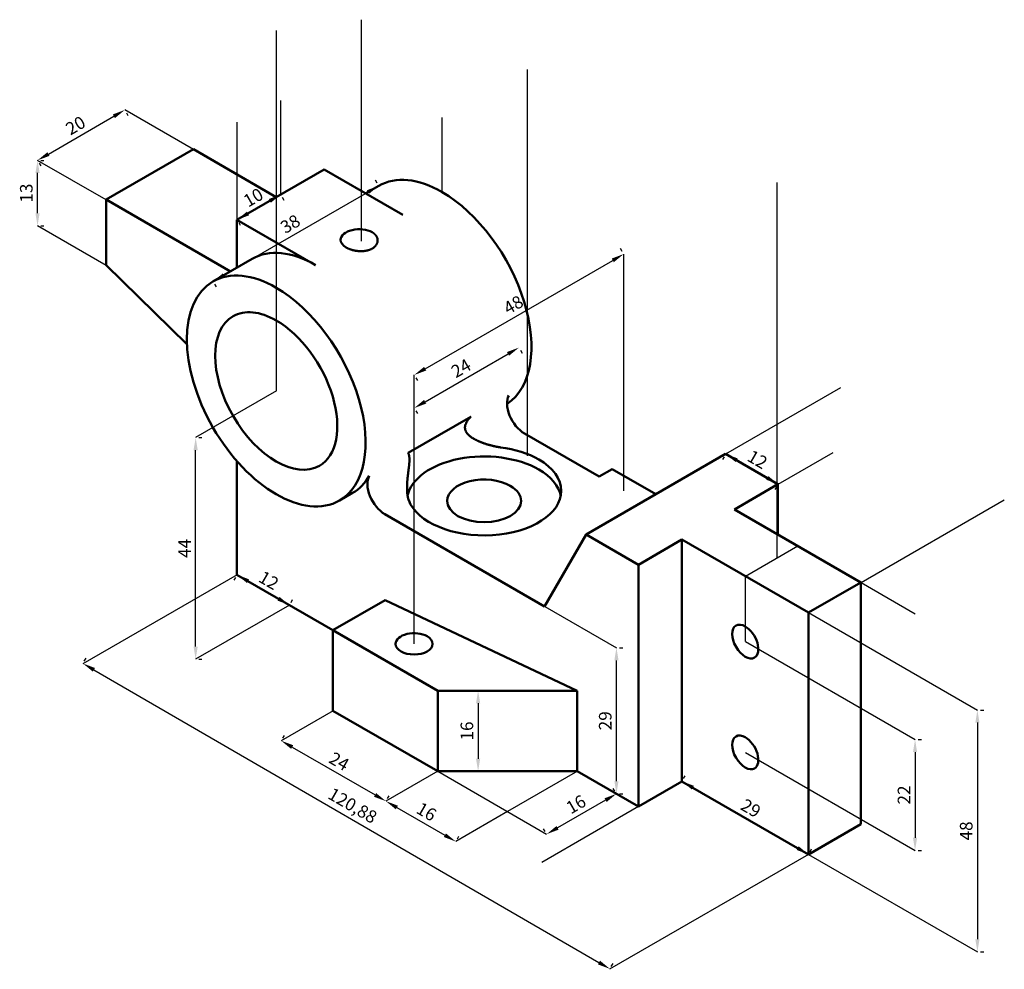
# Model space of a CAD drawing. Units: millimetres. Extents: x 3904 to 4099, y 5304 to 5492.
import ezdxf

# ---------------------------------------------------------------- set-up
doc = ezdxf.new("R2010")
doc.units = ezdxf.units.MM
doc.layers.add('M-DIMS', color=2, linetype='Continuous', lineweight=25)
doc.layers.add('M-OUTL', color=7, linetype='Continuous', lineweight=50)
doc.styles.get("Standard").update_dxf_attribs({"font": 'arial.ttf'})
doc.dimstyles.new('ISO-25', dxfattribs={"dimtxt": 2.5, "dimasz": 2.5, "dimexe": 1.25, "dimexo": 0.625, "dimtad": 1, "dimtxsty": 'Standard', "dimcen": 2.5, "dimadec": 0, "dimazin": 0, "dimtfac": 1, "dimtmove": 0, "dimatfit": 3, "dimfxl": 1, "dimarcsym": 0})

# ---------------------------------------------------------------- blocks, each defined once
blk = doc.blocks.new('*D1')
at = {"layer": 'Defpoints', "color": 0, "transparency": 16777216}
for p in [(4022.48, 5367.43), (4022.48, 5367.43), (4022.48, 5338.43)]:
    blk.add_point(p, dxfattribs=at)
at = {"layer": 'M-DIMS', "color": 0, "lineweight": -2, "transparency": 16777216}
for p, q in [((4023.11, 5367.43), (4023.73, 5367.43)), ((4022.48, 5340.93), (4022.48, 5364.93)), ((4023.11, 5338.43), (4023.73, 5338.43))]:
    blk.add_line(p, q, dxfattribs=at)
at = {"layer": 'M-DIMS', "color": 0, "transparency": 16777216}
for points in [[(4022.07, 5364.93), (4022.9, 5364.93), (4022.48, 5367.43)], [(4022.07, 5340.93), (4022.9, 5340.93), (4022.48, 5338.43)]]:
    blk.add_solid(points, dxfattribs=at)
at = {"layer": 'M-DIMS', "color": 0, "transparency": 16777216, "insert": (4020.58, 5352.93), "char_height": 2.5, "attachment_point": 5, "rotation": 90}
blk.add_mtext('29', dxfattribs=at)
blk = doc.blocks.new('*D2')
at = {"layer": 'Defpoints', "color": 0, "transparency": 16777216}
for p in [(3995.02, 5358.9), (3995.02, 5342.9), (3995.02, 5342.9)]:
    blk.add_point(p, dxfattribs=at)
at = {"layer": 'M-DIMS', "color": 0, "lineweight": -2, "transparency": 16777216}
for p, q in [((3995.65, 5358.9), (3996.27, 5358.9)), ((3995.02, 5356.4), (3995.02, 5345.4)), ((3995.65, 5342.9), (3996.27, 5342.9))]:
    blk.add_line(p, q, dxfattribs=at)
at = {"layer": 'M-DIMS', "color": 0, "transparency": 16777216}
for points in [[(3994.61, 5356.4), (3995.44, 5356.4), (3995.02, 5358.9)], [(3994.61, 5345.4), (3995.44, 5345.4), (3995.02, 5342.9)]]:
    blk.add_solid(points, dxfattribs=at)
at = {"layer": 'M-DIMS', "color": 0, "transparency": 16777216, "insert": (3993.12, 5350.9), "char_height": 2.5, "attachment_point": 5, "rotation": 90}
blk.add_mtext('16', dxfattribs=at)
blk = doc.blocks.new('*D3')
at = {"layer": 'Defpoints', "color": 0, "transparency": 16777216}
for p in [(4022.48, 5338.43), (4008.63, 5330.43), (4008.63, 5330.43)]:
    blk.add_point(p, dxfattribs=at)
at = {"layer": 'M-DIMS', "color": 0, "lineweight": -2, "transparency": 16777216}
for p, q in [((4022.17, 5338.97), (4021.86, 5339.51)), ((4020.32, 5337.18), (4010.79, 5331.68)), ((4008.32, 5330.97), (4008, 5331.51))]:
    blk.add_line(p, q, dxfattribs=at)
at = {"layer": 'M-DIMS', "color": 0, "transparency": 16777216}
for points in [[(4020.11, 5337.54), (4020.53, 5336.81), (4022.48, 5338.43)], [(4010.59, 5332.04), (4011, 5331.31), (4008.63, 5330.43)]]:
    blk.add_solid(points, dxfattribs=at)
at = {"layer": 'M-DIMS', "color": 0, "transparency": 16777216, "insert": (4014.61, 5336.07), "char_height": 2.5, "attachment_point": 5, "rotation": 30}
blk.add_mtext('16', dxfattribs=at)
blk = doc.blocks.new('*D4')
at = {"layer": 'Defpoints', "color": 0, "transparency": 16777216}
for p in [(4003.13, 5427.02), (4003.13, 5427.02), (3982.35, 5415.02)]:
    blk.add_point(p, dxfattribs=at)
at = {"layer": 'M-DIMS', "color": 0, "lineweight": -2, "transparency": 16777216}
for p, q in [((3984.51, 5416.27), (4000.97, 5425.77)), ((4003.44, 5426.48), (4003.76, 5425.94)), ((3982.66, 5414.48), (3982.97, 5413.94))]:
    blk.add_line(p, q, dxfattribs=at)
at = {"layer": 'M-DIMS', "color": 0, "transparency": 16777216}
for points in [[(4000.76, 5426.13), (4001.17, 5425.41), (4003.13, 5427.02)], [(3984.3, 5416.63), (3984.72, 5415.91), (3982.35, 5415.02)]]:
    blk.add_solid(points, dxfattribs=at)
at = {"layer": 'M-DIMS', "color": 0, "transparency": 16777216, "insert": (3991.8, 5422.65), "char_height": 2.5, "attachment_point": 5, "rotation": 30}
blk.add_mtext('24', dxfattribs=at)
blk = doc.blocks.new('*D5')
at = {"layer": 'Defpoints', "color": 0, "transparency": 16777216}
for p in [(4044.18, 5405.9), (4054.57, 5399.9), (4054.57, 5399.9)]:
    blk.add_point(p, dxfattribs=at)
at = {"layer": 'M-DIMS', "color": 0, "lineweight": -2, "transparency": 16777216}
for p, q in [((4043.87, 5405.36), (4043.56, 5404.82)), ((4046.35, 5404.65), (4052.41, 5401.15)), ((4054.26, 5399.36), (4053.95, 5398.82))]:
    blk.add_line(p, q, dxfattribs=at)
at = {"layer": 'M-DIMS', "color": 0, "transparency": 16777216}
for points in [[(4046.55, 5405.01), (4046.14, 5404.29), (4044.18, 5405.9)], [(4052.62, 5401.51), (4052.2, 5400.79), (4054.57, 5399.9)]]:
    blk.add_solid(points, dxfattribs=at)
at = {"layer": 'M-DIMS', "color": 0, "transparency": 16777216, "insert": (4050.32, 5404.53), "char_height": 2.5, "attachment_point": 5, "rotation": 330}
blk.add_mtext('12', dxfattribs=at)
blk = doc.blocks.new('*D6')
at = {"layer": 'Defpoints', "color": 0, "transparency": 16777216}
for p in [(3955.95, 5348.96), (3976.74, 5336.96), (3976.74, 5336.96)]:
    blk.add_point(p, dxfattribs=at)
at = {"layer": 'M-DIMS', "color": 0, "lineweight": -2, "transparency": 16777216}
for p, q in [((3956.27, 5349.5), (3956.58, 5350.04)), ((3958.12, 5347.71), (3974.57, 5338.21)), ((3977.05, 5337.5), (3977.36, 5338.04))]:
    blk.add_line(p, q, dxfattribs=at)
at = {"layer": 'M-DIMS', "color": 0, "transparency": 16777216}
for points in [[(3958.33, 5348.07), (3957.91, 5347.35), (3955.95, 5348.96)], [(3974.78, 5338.57), (3974.36, 5337.85), (3976.74, 5336.96)]]:
    blk.add_solid(points, dxfattribs=at)
at = {"layer": 'M-DIMS', "color": 0, "transparency": 16777216, "insert": (3967.29, 5344.59), "char_height": 2.5, "attachment_point": 5, "rotation": 330}
blk.add_mtext('24', dxfattribs=at)
blk = doc.blocks.new('*D7')
at = {"layer": 'Defpoints', "color": 0, "transparency": 16777216}
for p in [(3976.74, 5336.96), (3990.59, 5328.96), (3990.59, 5328.96)]:
    blk.add_point(p, dxfattribs=at)
at = {"layer": 'M-DIMS', "color": 0, "lineweight": -2, "transparency": 16777216}
for p, q in [((3977.05, 5337.5), (3977.36, 5338.04)), ((3978.9, 5335.71), (3988.43, 5330.21)), ((3990.91, 5329.5), (3991.22, 5330.04))]:
    blk.add_line(p, q, dxfattribs=at)
at = {"layer": 'M-DIMS', "color": 0, "transparency": 16777216}
for points in [[(3979.11, 5336.07), (3978.69, 5335.35), (3976.74, 5336.96)], [(3988.64, 5330.57), (3988.22, 5329.85), (3990.59, 5328.96)]]:
    blk.add_solid(points, dxfattribs=at)
at = {"layer": 'M-DIMS', "color": 0, "transparency": 16777216, "insert": (3984.62, 5334.61), "char_height": 2.5, "attachment_point": 5, "rotation": 330}
blk.add_mtext('16', dxfattribs=at)
blk = doc.blocks.new('*D8')
at = {"layer": 'Defpoints', "color": 0, "transparency": 16777216}
for p in [(3947.19, 5381.9), (3957.58, 5375.9), (3957.58, 5375.9)]:
    blk.add_point(p, dxfattribs=at)
at = {"layer": 'M-DIMS', "color": 0, "lineweight": -2, "transparency": 16777216}
for p, q in [((3946.87, 5381.36), (3946.56, 5380.82)), ((3949.35, 5380.65), (3955.41, 5377.15)), ((3957.89, 5376.44), (3958.2, 5376.98))]:
    blk.add_line(p, q, dxfattribs=at)
at = {"layer": 'M-DIMS', "color": 0, "transparency": 16777216}
for points in [[(3949.56, 5381.01), (3949.14, 5380.29), (3947.19, 5381.9)], [(3955.62, 5377.51), (3955.2, 5376.79), (3957.58, 5375.9)]]:
    blk.add_solid(points, dxfattribs=at)
at = {"layer": 'M-DIMS', "color": 0, "transparency": 16777216, "insert": (3953.32, 5380.53), "char_height": 2.5, "attachment_point": 5, "rotation": 330}
blk.add_mtext('12', dxfattribs=at)
blk = doc.blocks.new('*D9')
at = {"layer": 'Defpoints', "color": 0, "transparency": 16777216}
for p in [(3938.96, 5409.15), (3938.96, 5409.15), (3938.96, 5365.15)]:
    blk.add_point(p, dxfattribs=at)
at = {"layer": 'M-DIMS', "color": 0, "lineweight": -2, "transparency": 16777216}
for p, q in [((3939.58, 5409.15), (3940.21, 5409.15)), ((3938.96, 5367.65), (3938.96, 5406.65)), ((3939.58, 5365.15), (3940.21, 5365.15))]:
    blk.add_line(p, q, dxfattribs=at)
at = {"layer": 'M-DIMS', "color": 0, "transparency": 16777216}
for points in [[(3938.54, 5406.65), (3939.37, 5406.65), (3938.96, 5409.15)], [(3938.54, 5367.65), (3939.37, 5367.65), (3938.96, 5365.15)]]:
    blk.add_solid(points, dxfattribs=at)
at = {"layer": 'M-DIMS', "color": 0, "transparency": 16777216, "insert": (3937.08, 5387.15), "char_height": 2.5, "attachment_point": 5, "rotation": 90}
blk.add_mtext('44', dxfattribs=at)
blk = doc.blocks.new('*D10')
at = {"layer": 'Defpoints', "color": 0, "transparency": 16777216}
for p in [(3916.55, 5364.21), (4021.13, 5303.59), (4021.18, 5303.68)]:
    blk.add_point(p, dxfattribs=at)
at = {"layer": 'M-DIMS', "color": 0, "lineweight": -2, "transparency": 16777216}
for p, q in [((3916.86, 5364.75), (3917.23, 5365.38)), ((3918.76, 5363.05), (4019.02, 5304.93)), ((4021.44, 5304.13), (4021.81, 5304.76))]:
    blk.add_line(p, q, dxfattribs=at)
at = {"layer": 'M-DIMS', "color": 0, "transparency": 16777216}
for points in [[(3918.97, 5363.41), (3918.55, 5362.69), (3916.6, 5364.3)], [(4019.23, 5305.3), (4018.81, 5304.57), (4021.18, 5303.68)]]:
    blk.add_solid(points, dxfattribs=at)
at = {"layer": 'M-DIMS', "color": 0, "transparency": 16777216, "insert": (3969.96, 5335.83), "char_height": 2.5, "attachment_point": 5, "rotation": 329.9013}
blk.add_mtext('120,88', dxfattribs=at)
blk = doc.blocks.new('*D11')
at = {"layer": 'Defpoints', "color": 0, "transparency": 16777216}
for p in [(3907.57, 5464.19), (3907.57, 5464.19), (3907.57, 5451.19)]:
    blk.add_point(p, dxfattribs=at)
at = {"layer": 'M-DIMS', "color": 0, "lineweight": -2, "transparency": 16777216}
for p, q in [((3908.2, 5464.19), (3908.82, 5464.19)), ((3907.57, 5453.69), (3907.57, 5461.69)), ((3908.2, 5451.19), (3908.82, 5451.19))]:
    blk.add_line(p, q, dxfattribs=at)
at = {"layer": 'M-DIMS', "color": 0, "transparency": 16777216}
for points in [[(3907.16, 5461.69), (3907.99, 5461.69), (3907.57, 5464.19)], [(3907.16, 5453.69), (3907.99, 5453.69), (3907.57, 5451.19)]]:
    blk.add_solid(points, dxfattribs=at)
at = {"layer": 'M-DIMS', "color": 0, "transparency": 16777216, "insert": (3905.67, 5457.69), "char_height": 2.5, "attachment_point": 5, "rotation": 90}
blk.add_mtext('13', dxfattribs=at)
blk = doc.blocks.new('*D12')
at = {"layer": 'Defpoints', "color": 0, "transparency": 16777216}
for p in [(3924.89, 5474.19), (3924.89, 5474.19), (3907.57, 5464.19)]:
    blk.add_point(p, dxfattribs=at)
at = {"layer": 'M-DIMS', "color": 0, "lineweight": -2, "transparency": 16777216}
for p, q in [((3909.74, 5465.44), (3922.73, 5472.94)), ((3925.21, 5473.65), (3925.52, 5473.11)), ((3907.89, 5463.65), (3908.2, 5463.11))]:
    blk.add_line(p, q, dxfattribs=at)
at = {"layer": 'M-DIMS', "color": 0, "transparency": 16777216}
for points in [[(3922.52, 5473.3), (3922.94, 5472.58), (3924.89, 5474.19)], [(3909.53, 5465.8), (3909.95, 5465.08), (3907.57, 5464.19)]]:
    blk.add_solid(points, dxfattribs=at)
at = {"layer": 'M-DIMS', "color": 0, "transparency": 16777216, "insert": (3915.28, 5470.84), "char_height": 2.5, "attachment_point": 5, "rotation": 30}
blk.add_mtext('20', dxfattribs=at)
blk = doc.blocks.new('*D13')
at = {"layer": 'Defpoints', "color": 0, "transparency": 16777216}
for p in [(3955.85, 5457.39), (3955.85, 5457.39), (3947.19, 5452.39)]:
    blk.add_point(p, dxfattribs=at)
at = {"layer": 'M-DIMS', "color": 0, "lineweight": -2, "transparency": 16777216}
for p, q in [((3956.16, 5456.85), (3956.47, 5456.31)), ((3949.35, 5453.64), (3953.68, 5456.14)), ((3947.5, 5451.85), (3947.81, 5451.31))]:
    blk.add_line(p, q, dxfattribs=at)
at = {"layer": 'M-DIMS', "color": 0, "transparency": 16777216}
for points in [[(3953.47, 5456.51), (3953.89, 5455.78), (3955.85, 5457.39)], [(3949.14, 5454.01), (3949.56, 5453.28), (3947.19, 5452.39)]]:
    blk.add_solid(points, dxfattribs=at)
at = {"layer": 'M-DIMS', "color": 0, "transparency": 16777216, "insert": (3950.56, 5456.54), "char_height": 2.5, "attachment_point": 5, "rotation": 30}
blk.add_mtext('10', dxfattribs=at)
blk = doc.blocks.new('*D14')
at = {"layer": 'Defpoints', "color": 0, "transparency": 16777216}
for p in [(3975.31, 5459.14), (3975.31, 5459.14), (3942.4, 5440.14)]:
    blk.add_point(p, dxfattribs=at)
at = {"layer": 'M-DIMS', "color": 0, "lineweight": -2, "transparency": 16777216}
for p, q in [((3975, 5459.68), (3974.68, 5460.23)), ((3944.57, 5441.39), (3973.14, 5457.89)), ((3942.71, 5439.6), (3943.03, 5439.06))]:
    blk.add_line(p, q, dxfattribs=at)
at = {"layer": 'M-DIMS', "color": 0, "transparency": 16777216}
for points in [[(3972.94, 5458.25), (3973.35, 5457.53), (3975.31, 5459.14)], [(3944.36, 5441.75), (3944.77, 5441.03), (3942.4, 5440.14)]]:
    blk.add_solid(points, dxfattribs=at)
at = {"layer": 'M-DIMS', "color": 0, "transparency": 16777216, "insert": (3957.9, 5451.29), "char_height": 2.5, "attachment_point": 5, "rotation": 30}
blk.add_mtext('38', dxfattribs=at)
blk = doc.blocks.new('*D15')
at = {"layer": 'Defpoints', "color": 0, "transparency": 16777216}
for p in [(4023.92, 5445.58), (4023.92, 5445.58), (3982.35, 5421.58)]:
    blk.add_point(p, dxfattribs=at)
at = {"layer": 'M-DIMS', "color": 0, "lineweight": -2, "transparency": 16777216}
for p, q in [((4023.6, 5446.12), (4023.29, 5446.67)), ((3984.51, 5422.83), (4021.75, 5444.33)), ((3982.66, 5421.04), (3982.97, 5420.5))]:
    blk.add_line(p, q, dxfattribs=at)
at = {"layer": 'M-DIMS', "color": 0, "transparency": 16777216}
for points in [[(4021.54, 5444.69), (4021.96, 5443.97), (4023.92, 5445.58)], [(3984.3, 5423.19), (3984.72, 5422.47), (3982.35, 5421.58)]]:
    blk.add_solid(points, dxfattribs=at)
at = {"layer": 'M-DIMS', "color": 0, "transparency": 16777216, "insert": (4002.18, 5435.23), "char_height": 2.5, "attachment_point": 5, "rotation": 30}
blk.add_mtext('48', dxfattribs=at)
blk = doc.blocks.new('*D16')
at = {"layer": 'Defpoints', "color": 0, "transparency": 16777216}
for p in [(4094.13, 5355.06), (4094.13, 5307.06), (4094.13, 5307.06)]:
    blk.add_point(p, dxfattribs=at)
at = {"layer": 'M-DIMS', "color": 0, "lineweight": -2, "transparency": 16777216}
for p, q in [((4094.76, 5355.06), (4095.38, 5355.06)), ((4094.13, 5352.56), (4094.13, 5309.56)), ((4094.76, 5307.06), (4095.38, 5307.06))]:
    blk.add_line(p, q, dxfattribs=at)
at = {"layer": 'M-DIMS', "color": 0, "transparency": 16777216}
for points in [[(4093.72, 5352.56), (4094.55, 5352.56), (4094.13, 5355.06)], [(4093.72, 5309.56), (4094.55, 5309.56), (4094.13, 5307.06)]]:
    blk.add_solid(points, dxfattribs=at)
at = {"layer": 'M-DIMS', "color": 0, "transparency": 16777216, "insert": (4092.23, 5331.06), "char_height": 2.5, "attachment_point": 5, "rotation": 90}
blk.add_mtext('48', dxfattribs=at)
blk = doc.blocks.new('*D17')
at = {"layer": 'Defpoints', "color": 0, "transparency": 16777216}
for p in [(4081.76, 5349.2), (4081.76, 5327.2), (4081.76, 5327.2)]:
    blk.add_point(p, dxfattribs=at)
at = {"layer": 'M-DIMS', "color": 0, "lineweight": -2, "transparency": 16777216}
for p, q in [((4082.38, 5349.2), (4083.01, 5349.2)), ((4081.76, 5346.7), (4081.76, 5329.7)), ((4082.38, 5327.2), (4083.01, 5327.2))]:
    blk.add_line(p, q, dxfattribs=at)
at = {"layer": 'M-DIMS', "color": 0, "transparency": 16777216}
for points in [[(4081.34, 5346.7), (4082.17, 5346.7), (4081.76, 5349.2)], [(4081.34, 5329.7), (4082.17, 5329.7), (4081.76, 5327.2)]]:
    blk.add_solid(points, dxfattribs=at)
at = {"layer": 'M-DIMS', "color": 0, "transparency": 16777216, "insert": (4079.88, 5338.2), "char_height": 2.5, "attachment_point": 5, "rotation": 90}
blk.add_mtext('22', dxfattribs=at)
blk = doc.blocks.new('*D18')
at = {"layer": 'Defpoints', "color": 0, "transparency": 16777216}
for p in [(4035.49, 5340.9), (4060.61, 5326.4), (4060.61, 5326.4)]:
    blk.add_point(p, dxfattribs=at)
at = {"layer": 'M-DIMS', "color": 0, "lineweight": -2, "transparency": 16777216}
for p, q in [((4035.81, 5341.44), (4036.12, 5341.98)), ((4037.66, 5339.65), (4058.44, 5327.65)), ((4060.92, 5326.94), (4061.23, 5327.48))]:
    blk.add_line(p, q, dxfattribs=at)
at = {"layer": 'M-DIMS', "color": 0, "transparency": 16777216}
for points in [[(4037.87, 5340.01), (4037.45, 5339.29), (4035.49, 5340.9)], [(4058.65, 5328.01), (4058.24, 5327.29), (4060.61, 5326.4)]]:
    blk.add_solid(points, dxfattribs=at)
at = {"layer": 'M-DIMS', "color": 0, "transparency": 16777216, "insert": (4049, 5335.3), "char_height": 2.5, "attachment_point": 5, "rotation": 330}
blk.add_mtext('29', dxfattribs=at)

msp = doc.modelspace()

# ---------------------------------------------------------------- linework, layer by layer
at = {"layer": 'M-DIMS'}
for p, q in [((3971.857, 5448.15), (3971.857, 5492.113)), ((3954.98, 5489.032), (3954.98, 5489.941)), ((3954.98, 5418.4), (3954.98, 5489.032)), ((4004.766, 5482.215), (4004.766, 5405.498)), ((3955.846, 5457.394), (3955.846, 5476.095)), ((3938.525, 5466.319), (3924.895, 5474.188)), ((3987.889, 5457.9), (3987.889, 5472.716)), ((3947.185, 5452.394), (3947.185, 5471.743)), ((3921.205, 5456.319), (3907.574, 5464.188)), ((4054.412, 5385.307), (4054.412, 5459.809)), ((3921.205, 5443.319), (3907.574, 5451.188)), ((4023.915, 5445.583), (4023.915, 5398.6)), ((3982.346, 5368.2), (3982.346, 5421.583)), ((3954.98, 5418.4), (3938.957, 5409.149)), ((4044.18, 5405.9), (4067.001, 5419.075)), ((4054.573, 5399.9), (4065.471, 5406.192)), ((4071.027, 5380.4), (4099.471, 5396.822)), ((4048.077, 5381.65), (4058.47, 5387.65)), ((3947.185, 5381.9), (3916.547, 5364.211)), ((4048.077, 5368.65), (4048.077, 5381.65)), ((4071.027, 5380.4), (4081.805, 5374.178)), ((3957.578, 5375.9), (3938.957, 5365.149)), ((4008.24, 5375.65), (4022.485, 5367.426)), ((4060.635, 5374.4), (4094.132, 5355.06)), ((4048.077, 5368.65), (4081.758, 5349.204)), ((3966.238, 5354.9), (3955.954, 5348.962)), ((4048.077, 5346.65), (4081.758, 5327.204)), ((3987.023, 5342.9), (3976.738, 5336.962)), ((3987.023, 5342.9), (4008.628, 5330.426)), ((4014.735, 5342.9), (4000.879, 5334.9)), ((4026.86, 5335.9), (4007.68, 5324.826)), ((4000.879, 5334.9), (3990.595, 5328.962)), ((4060.635, 5326.4), (4021.128, 5303.591)), ((4060.635, 5326.4), (4094.132, 5307.06))]:
    msp.add_line(p, q, dxfattribs=at)
at = {"layer": 'M-OUTL'}
for p, q in [((3921.179, 5456.4), (3938.5, 5466.4)), ((3938.5, 5466.4), (3954.954, 5456.9)), ((3947.16, 5452.4), (3964.481, 5462.4)), ((3980.069, 5453.4), (3964.481, 5462.4)), ((3972.715, 5457.646), (3975.31, 5459.144)), ((3921.179, 5456.4), (3945.869, 5442.146)), ((3921.179, 5443.4), (3921.179, 5456.4)), ((3962.749, 5443.4), (3947.16, 5452.4)), ((3947.16, 5442.891), (3947.16, 5452.4)), ((3937.219, 5427.708), (3921.179, 5443.4)), ((3942.401, 5440.144), (3950.195, 5444.644)), ((3981.141, 5406.1), (3993.579, 5413.281)), ((4019.04, 5401.4), (4004.224, 5409.954)), ((4016.442, 5389.9), (4044.155, 5405.9)), ((4054.547, 5399.9), (4044.155, 5405.9)), ((3947.16, 5381.9), (3947.16, 5404.481)), ((4019.04, 5401.4), (4021.638, 5402.9)), ((4030.299, 5397.9), (4021.638, 5402.9)), ((3967.508, 5396.656), (3970.106, 5398.156)), ((4045.887, 5394.9), (4054.547, 5399.9)), ((4054.547, 5389.9), (4054.547, 5399.9)), ((4071.002, 5380.4), (4045.887, 5394.9)), ((4008.215, 5375.65), (3976.511, 5393.954)), ((4016.442, 5389.9), (4008.215, 5375.65)), ((4026.835, 5383.9), (4016.442, 5389.9)), ((4026.835, 5383.9), (4035.495, 5388.9)), ((4060.61, 5374.4), (4035.495, 5388.9)), ((4035.495, 5340.9), (4035.495, 5388.9)), ((4026.835, 5335.9), (4026.835, 5383.9)), ((3947.16, 5381.9), (3966.213, 5370.9)), ((4060.61, 5374.4), (4071.002, 5380.4)), ((4071.002, 5332.4), (4071.002, 5380.4)), ((3966.213, 5370.9), (3976.605, 5376.9)), ((3976.605, 5376.9), (4014.71, 5358.9)), ((4060.61, 5326.4), (4060.61, 5374.4)), ((3966.213, 5354.9), (3966.213, 5370.9)), ((3986.997, 5358.9), (3966.213, 5370.9)), ((3986.997, 5342.9), (3986.997, 5358.9)), ((4014.71, 5358.9), (3986.997, 5358.9)), ((4014.71, 5350.9), (4014.71, 5358.9)), ((3986.997, 5342.9), (3966.213, 5354.9)), ((4014.71, 5342.9), (4014.71, 5350.9)), ((4014.71, 5342.9), (3986.997, 5342.9)), ((4014.71, 5342.9), (4026.835, 5335.9)), ((4026.835, 5335.9), (4035.495, 5340.9)), ((4060.61, 5326.4), (4035.495, 5340.9)), ((4060.61, 5326.4), (4071.002, 5332.4))]:
    msp.add_line(p, q, dxfattribs=at)
for points in [[(3975.083, 5448.29), (3975.083, 5448.307), (3975.083, 5448.324), (3975.082, 5448.341), (3975.082, 5448.358), (3975.081, 5448.376), (3975.08, 5448.393), (3975.078, 5448.41), (3975.077, 5448.428), (3975.075, 5448.445), (3975.073, 5448.463), (3975.071, 5448.48), (3975.069, 5448.498), (3975.066, 5448.515), (3975.063, 5448.533), (3975.06, 5448.551), (3975.057, 5448.568), (3975.054, 5448.586), (3975.05, 5448.604), (3975.046, 5448.621), (3975.042, 5448.639), (3975.038, 5448.657), (3975.033, 5448.675), (3975.028, 5448.693), (3975.023, 5448.711), (3975.018, 5448.728), (3975.012, 5448.746), (3975.007, 5448.764), (3975.001, 5448.782), (3974.995, 5448.8), (3974.988, 5448.818), (3974.981, 5448.836), (3974.975, 5448.854), (3974.967, 5448.871), (3974.96, 5448.889), (3974.952, 5448.907), (3974.944, 5448.925), (3974.936, 5448.943), (3974.928, 5448.961), (3974.919, 5448.979), (3974.91, 5448.996), (3974.901, 5449.014), (3974.892, 5449.032), (3974.882, 5449.05), (3974.872, 5449.067), (3974.862, 5449.085), (3974.852, 5449.103), (3974.841, 5449.12), (3974.83, 5449.138), (3974.819, 5449.155), (3974.808, 5449.173), (3974.796, 5449.19), (3974.784, 5449.208), (3974.772, 5449.225), (3974.76, 5449.242), (3974.747, 5449.26), (3974.734, 5449.277), (3974.721, 5449.294), (3974.708, 5449.311), (3974.694, 5449.328), (3974.68, 5449.345), (3974.666, 5449.362), (3974.652, 5449.379), (3974.637, 5449.396), (3974.622, 5449.412), (3974.607, 5449.429), (3974.591, 5449.446), (3974.575, 5449.462), (3974.559, 5449.479), (3974.543, 5449.495), (3974.527, 5449.511), (3974.51, 5449.527), (3974.493, 5449.544), (3974.476, 5449.56), (3974.458, 5449.576), (3974.44, 5449.591), (3974.422, 5449.607), (3974.404, 5449.623), (3974.385, 5449.638), (3974.366, 5449.654), (3974.347, 5449.669), (3974.328, 5449.685), (3974.308, 5449.7), (3974.288, 5449.715), (3974.268, 5449.73), (3974.248, 5449.745), (3974.227, 5449.759), (3974.206, 5449.774), (3974.185, 5449.788), (3974.164, 5449.803), (3974.142, 5449.817), (3974.12, 5449.831), (3974.098, 5449.845), (3974.076, 5449.859), (3974.053, 5449.873), (3974.03, 5449.886), (3974.007, 5449.9)], [(3968.811, 5446.9), (3968.892, 5446.854), (3968.975, 5446.81), (3969.06, 5446.767), (3969.147, 5446.725), (3969.235, 5446.685), (3969.325, 5446.646), (3969.417, 5446.608), (3969.51, 5446.571), (3969.604, 5446.536), (3969.699, 5446.503), (3969.795, 5446.471), (3969.892, 5446.441), (3969.989, 5446.412), (3970.086, 5446.385), (3970.184, 5446.359), (3970.282, 5446.335), (3970.38, 5446.313), (3970.478, 5446.292), (3970.575, 5446.273), (3970.672, 5446.255), (3970.769, 5446.239), (3970.865, 5446.224), (3970.96, 5446.211), (3971.055, 5446.2), (3971.15, 5446.189), (3971.243, 5446.181), (3971.337, 5446.173), (3971.429, 5446.167), (3971.521, 5446.163), (3971.612, 5446.16), (3971.702, 5446.158), (3971.792, 5446.157), (3971.88, 5446.158), (3971.968, 5446.16), (3972.055, 5446.163), (3972.141, 5446.168), (3972.226, 5446.174), (3972.31, 5446.181), (3972.394, 5446.189), (3972.476, 5446.199), (3972.557, 5446.209), (3972.637, 5446.221), (3972.716, 5446.234), (3972.795, 5446.248), (3972.872, 5446.263), (3972.948, 5446.28), (3973.023, 5446.297), (3973.097, 5446.315), (3973.17, 5446.335), (3973.242, 5446.356), (3973.312, 5446.377), (3973.382, 5446.4), (3973.45, 5446.424), (3973.518, 5446.449), (3973.584, 5446.475), (3973.649, 5446.501), (3973.713, 5446.529), (3973.775, 5446.558), (3973.837, 5446.588), (3973.897, 5446.619), (3973.956, 5446.65), (3974.014, 5446.683), (3974.07, 5446.717), (3974.125, 5446.751), (3974.179, 5446.787), (3974.232, 5446.823), (3974.283, 5446.86), (3974.333, 5446.899), (3974.381, 5446.938), (3974.428, 5446.978), (3974.474, 5447.018), (3974.518, 5447.06), (3974.561, 5447.103), (3974.603, 5447.146), (3974.642, 5447.19), (3974.681, 5447.235), (3974.718, 5447.281), (3974.753, 5447.328), (3974.787, 5447.375), (3974.819, 5447.423), (3974.849, 5447.472), (3974.878, 5447.522), (3974.905, 5447.573), (3974.93, 5447.624), (3974.954, 5447.676), (3974.975, 5447.728), (3974.995, 5447.782), (3975.013, 5447.836), (3975.029, 5447.89), (3975.043, 5447.946), (3975.055, 5448.002), (3975.065, 5448.058), (3975.073, 5448.115), (3975.079, 5448.173), (3975.082, 5448.231), (3975.083, 5448.29)], [(3999.474, 5407.212), (3999.336, 5407.23), (3999.198, 5407.25), (3999.061, 5407.271), (3998.923, 5407.293), (3998.787, 5407.317), (3998.65, 5407.342), (3998.515, 5407.368), (3998.38, 5407.396), (3998.245, 5407.424), (3998.112, 5407.454), (3997.979, 5407.484), (3997.848, 5407.515), (3997.717, 5407.548), (3997.587, 5407.581), (3997.458, 5407.615), (3997.33, 5407.65), (3997.202, 5407.686), (3997.076, 5407.722), (3996.951, 5407.759), (3996.827, 5407.797), (3996.704, 5407.836), (3996.582, 5407.875), (3996.461, 5407.915), (3996.341, 5407.956), (3996.222, 5407.997), (3996.104, 5408.039), (3995.988, 5408.081), (3995.872, 5408.124), (3995.758, 5408.168), (3995.645, 5408.213), (3995.533, 5408.258), (3995.422, 5408.303), (3995.312, 5408.349), (3995.204, 5408.396), (3995.097, 5408.444), (3994.991, 5408.492), (3994.886, 5408.541), (3994.783, 5408.59), (3994.681, 5408.64), (3994.58, 5408.691), (3994.48, 5408.743), (3994.382, 5408.795), (3994.286, 5408.848), (3994.191, 5408.902), (3994.097, 5408.957), (3994.005, 5409.012), (3993.914, 5409.069), (3993.825, 5409.126), (3993.738, 5409.185), (3993.653, 5409.244), (3993.569, 5409.304), (3993.487, 5409.366), (3993.408, 5409.428), (3993.33, 5409.492), (3993.255, 5409.557), (3993.181, 5409.623), (3993.11, 5409.69), (3993.042, 5409.759), (3992.976, 5409.829), (3992.913, 5409.901), (3992.853, 5409.974), (3992.796, 5410.048), (3992.743, 5410.125), (3992.692, 5410.202), (3992.646, 5410.282), (3992.603, 5410.363), (3992.564, 5410.445), (3992.529, 5410.53), (3992.499, 5410.615), (3992.473, 5410.703), (3992.452, 5410.791), (3992.435, 5410.881), (3992.424, 5410.972), (3992.417, 5411.065), (3992.416, 5411.158), (3992.42, 5411.251), (3992.428, 5411.346), (3992.442, 5411.44), (3992.46, 5411.535), (3992.484, 5411.63), (3992.512, 5411.724), (3992.544, 5411.819), (3992.581, 5411.913), (3992.621, 5412.006), (3992.666, 5412.099), (3992.715, 5412.191), (3992.766, 5412.282), (3992.822, 5412.372), (3992.88, 5412.461), (3992.941, 5412.549), (3993.006, 5412.636), (3993.073, 5412.722), (3993.142, 5412.807), (3993.214, 5412.891), (3993.288, 5412.973), (3993.365, 5413.055)], [(3993.579, 5413.281), (3993.577, 5413.279), (3993.575, 5413.277), (3993.573, 5413.274), (3993.57, 5413.272), (3993.568, 5413.269), (3993.566, 5413.267), (3993.564, 5413.265), (3993.562, 5413.262), (3993.559, 5413.26), (3993.557, 5413.258), (3993.555, 5413.255), (3993.553, 5413.253), (3993.551, 5413.25), (3993.548, 5413.248), (3993.546, 5413.246), (3993.544, 5413.243), (3993.542, 5413.241), (3993.539, 5413.239), (3993.537, 5413.236), (3993.535, 5413.234), (3993.533, 5413.232), (3993.531, 5413.229), (3993.528, 5413.227), (3993.526, 5413.224), (3993.524, 5413.222), (3993.522, 5413.22), (3993.519, 5413.217), (3993.517, 5413.215), (3993.515, 5413.213), (3993.513, 5413.21), (3993.511, 5413.208), (3993.508, 5413.206), (3993.506, 5413.203), (3993.504, 5413.201), (3993.502, 5413.198), (3993.499, 5413.196), (3993.497, 5413.194), (3993.495, 5413.191), (3993.493, 5413.189), (3993.491, 5413.187), (3993.488, 5413.184), (3993.486, 5413.182), (3993.484, 5413.18), (3993.482, 5413.177), (3993.479, 5413.175), (3993.477, 5413.172), (3993.475, 5413.17), (3993.473, 5413.168), (3993.471, 5413.165), (3993.468, 5413.163), (3993.466, 5413.161), (3993.464, 5413.158), (3993.462, 5413.156), (3993.459, 5413.154), (3993.457, 5413.151), (3993.455, 5413.149), (3993.453, 5413.146), (3993.45, 5413.144), (3993.448, 5413.142), (3993.446, 5413.139), (3993.444, 5413.137), (3993.441, 5413.135), (3993.439, 5413.132), (3993.437, 5413.13), (3993.435, 5413.128), (3993.432, 5413.125), (3993.43, 5413.123), (3993.428, 5413.121), (3993.426, 5413.118), (3993.424, 5413.116), (3993.421, 5413.113), (3993.419, 5413.111), (3993.417, 5413.109), (3993.415, 5413.106), (3993.412, 5413.104), (3993.41, 5413.102), (3993.408, 5413.099), (3993.406, 5413.097), (3993.403, 5413.095), (3993.401, 5413.092), (3993.399, 5413.09), (3993.397, 5413.088), (3993.394, 5413.085), (3993.392, 5413.083), (3993.39, 5413.081), (3993.388, 5413.078), (3993.385, 5413.076), (3993.383, 5413.073), (3993.381, 5413.071), (3993.378, 5413.069), (3993.376, 5413.066), (3993.374, 5413.064), (3993.372, 5413.062), (3993.369, 5413.059), (3993.367, 5413.057), (3993.365, 5413.055)], [(3980.911, 5399.159), (3980.911, 5399.24), (3980.912, 5399.322), (3980.913, 5399.404), (3980.915, 5399.486), (3980.917, 5399.568), (3980.92, 5399.651), (3980.923, 5399.734), (3980.926, 5399.817), (3980.93, 5399.9), (3980.934, 5399.984), (3980.939, 5400.067), (3980.944, 5400.151), (3980.95, 5400.235), (3980.955, 5400.319), (3980.962, 5400.404), (3980.968, 5400.488), (3980.975, 5400.573), (3980.982, 5400.658), (3980.99, 5400.743), (3980.997, 5400.828), (3981.005, 5400.913), (3981.014, 5400.998), (3981.022, 5401.084), (3981.031, 5401.17), (3981.04, 5401.255), (3981.049, 5401.341), (3981.059, 5401.427), (3981.069, 5401.513), (3981.079, 5401.599), (3981.089, 5401.685), (3981.099, 5401.772), (3981.109, 5401.858), (3981.12, 5401.944), (3981.13, 5402.031), (3981.141, 5402.117), (3981.152, 5402.204), (3981.163, 5402.29), (3981.173, 5402.377), (3981.184, 5402.463), (3981.195, 5402.55), (3981.206, 5402.636), (3981.217, 5402.723), (3981.228, 5402.809), (3981.238, 5402.895), (3981.249, 5402.981), (3981.259, 5403.067), (3981.27, 5403.153), (3981.28, 5403.238), (3981.289, 5403.324), (3981.299, 5403.409), (3981.308, 5403.493), (3981.317, 5403.578), (3981.326, 5403.662), (3981.334, 5403.745), (3981.342, 5403.828), (3981.349, 5403.91), (3981.356, 5403.992), (3981.362, 5404.072), (3981.368, 5404.152), (3981.373, 5404.231), (3981.378, 5404.309), (3981.382, 5404.386), (3981.385, 5404.462), (3981.388, 5404.536), (3981.39, 5404.609), (3981.391, 5404.681), (3981.392, 5404.751), (3981.391, 5404.82), (3981.391, 5404.887), (3981.389, 5404.952), (3981.387, 5405.016), (3981.384, 5405.077), (3981.38, 5405.137), (3981.376, 5405.195), (3981.371, 5405.251), (3981.366, 5405.306), (3981.36, 5405.358), (3981.353, 5405.408), (3981.346, 5405.457), (3981.339, 5405.503), (3981.331, 5405.548), (3981.322, 5405.591), (3981.313, 5405.632), (3981.304, 5405.672), (3981.295, 5405.709), (3981.285, 5405.745), (3981.275, 5405.78), (3981.265, 5405.812), (3981.255, 5405.843), (3981.245, 5405.873), (3981.234, 5405.901), (3981.223, 5405.928), (3981.213, 5405.953), (3981.202, 5405.976), (3981.191, 5405.999), (3981.18, 5406.02)], [(3981.18, 5406.02), (3981.179, 5406.02), (3981.179, 5406.021), (3981.179, 5406.022), (3981.178, 5406.023), (3981.178, 5406.024), (3981.177, 5406.024), (3981.177, 5406.025), (3981.176, 5406.026), (3981.176, 5406.027), (3981.176, 5406.028), (3981.175, 5406.028), (3981.175, 5406.029), (3981.174, 5406.03), (3981.174, 5406.031), (3981.174, 5406.032), (3981.173, 5406.032), (3981.173, 5406.033), (3981.172, 5406.034), (3981.172, 5406.035), (3981.171, 5406.036), (3981.171, 5406.037), (3981.171, 5406.037), (3981.17, 5406.038), (3981.17, 5406.039), (3981.169, 5406.04), (3981.169, 5406.041), (3981.168, 5406.041), (3981.168, 5406.042), (3981.168, 5406.043), (3981.167, 5406.044), (3981.167, 5406.045), (3981.166, 5406.046), (3981.166, 5406.046), (3981.166, 5406.047), (3981.165, 5406.048), (3981.165, 5406.049), (3981.164, 5406.05), (3981.164, 5406.051), (3981.164, 5406.051), (3981.163, 5406.052), (3981.163, 5406.053), (3981.162, 5406.054), (3981.162, 5406.055), (3981.161, 5406.056), (3981.161, 5406.056), (3981.161, 5406.057), (3981.16, 5406.058), (3981.16, 5406.059), (3981.159, 5406.06), (3981.159, 5406.061), (3981.159, 5406.061), (3981.158, 5406.062), (3981.158, 5406.063), (3981.157, 5406.064), (3981.157, 5406.065), (3981.157, 5406.066), (3981.156, 5406.066), (3981.156, 5406.067), (3981.155, 5406.068), (3981.155, 5406.069), (3981.155, 5406.07), (3981.154, 5406.071), (3981.154, 5406.072), (3981.153, 5406.072), (3981.153, 5406.073), (3981.153, 5406.074), (3981.152, 5406.075), (3981.152, 5406.076), (3981.151, 5406.077), (3981.151, 5406.077), (3981.151, 5406.078), (3981.15, 5406.079), (3981.15, 5406.08), (3981.149, 5406.081), (3981.149, 5406.082), (3981.149, 5406.083), (3981.148, 5406.083), (3981.148, 5406.084), (3981.147, 5406.085), (3981.147, 5406.086), (3981.147, 5406.087), (3981.146, 5406.088), (3981.146, 5406.089), (3981.145, 5406.09), (3981.145, 5406.09), (3981.145, 5406.091), (3981.144, 5406.092), (3981.144, 5406.093), (3981.144, 5406.094), (3981.143, 5406.095), (3981.143, 5406.096), (3981.142, 5406.096), (3981.142, 5406.097), (3981.142, 5406.098), (3981.141, 5406.099), (3981.141, 5406.1)], [(3981.261, 5396.696), (3981.253, 5396.717), (3981.246, 5396.738), (3981.238, 5396.759), (3981.23, 5396.781), (3981.223, 5396.802), (3981.216, 5396.824), (3981.208, 5396.846), (3981.201, 5396.868), (3981.194, 5396.89), (3981.187, 5396.912), (3981.18, 5396.934), (3981.174, 5396.957), (3981.167, 5396.979), (3981.16, 5397.002), (3981.154, 5397.025), (3981.148, 5397.048), (3981.141, 5397.071), (3981.135, 5397.094), (3981.129, 5397.117), (3981.123, 5397.141), (3981.117, 5397.164), (3981.111, 5397.188), (3981.105, 5397.212), (3981.1, 5397.236), (3981.094, 5397.26), (3981.089, 5397.284), (3981.083, 5397.308), (3981.078, 5397.332), (3981.073, 5397.357), (3981.068, 5397.381), (3981.063, 5397.406), (3981.058, 5397.431), (3981.053, 5397.455), (3981.048, 5397.48), (3981.044, 5397.505), (3981.039, 5397.53), (3981.035, 5397.556), (3981.03, 5397.581), (3981.026, 5397.606), (3981.022, 5397.632), (3981.017, 5397.657), (3981.013, 5397.683), (3981.009, 5397.708), (3981.006, 5397.734), (3981.002, 5397.76), (3980.998, 5397.786), (3980.994, 5397.812), (3980.991, 5397.838), (3980.988, 5397.864), (3980.984, 5397.89), (3980.981, 5397.917), (3980.978, 5397.943), (3980.975, 5397.969), (3980.971, 5397.996), (3980.969, 5398.023), (3980.966, 5398.049), (3980.963, 5398.076), (3980.96, 5398.103), (3980.957, 5398.129), (3980.955, 5398.156), (3980.952, 5398.183), (3980.95, 5398.21), (3980.948, 5398.237), (3980.945, 5398.264), (3980.943, 5398.292), (3980.941, 5398.319), (3980.939, 5398.346), (3980.937, 5398.373), (3980.935, 5398.401), (3980.934, 5398.428), (3980.932, 5398.456), (3980.93, 5398.483), (3980.929, 5398.511), (3980.927, 5398.539), (3980.926, 5398.566), (3980.924, 5398.594), (3980.923, 5398.622), (3980.922, 5398.65), (3980.921, 5398.678), (3980.919, 5398.706), (3980.918, 5398.734), (3980.918, 5398.762), (3980.917, 5398.79), (3980.916, 5398.818), (3980.915, 5398.846), (3980.914, 5398.874), (3980.914, 5398.903), (3980.913, 5398.931), (3980.913, 5398.959), (3980.912, 5398.988), (3980.912, 5399.016), (3980.912, 5399.045), (3980.912, 5399.073), (3980.911, 5399.102), (3980.911, 5399.13), (3980.911, 5399.159)]]:
    msp.add_lwpolyline(points, dxfattribs=at)
for centre, major_axis, start_param, end_param in [((3987.863, 5437.4), (12.554, -21.744), 2.3561945, 3.1415927), ((3987.863, 5437.4), (12.554, -21.744), 0.0277801, 2.3561945), ((3971.409, 5448.4), (3.674, 0), 0.7853982, 3.1415927), ((3971.409, 5448.4), (3.674, 0), 3.1415927, 3.9269908), ((3962.749, 5422.9), (12.554, -21.744), 2.3561945, 3.1415927), ((3954.954, 5418.4), (12.554, -21.744), 2.3561945, 3.1415927), ((3954.954, 5418.4), (12.554, -21.744), 3.1415927, 6.2831853), ((3954.954, 5418.4), (12.554, -21.744), 0, 2.3561945), ((3954.954, 5418.4), (8.573, -14.849), 3.1415927, 6.2831853), ((3954.954, 5418.4), (8.573, -14.849), 2.3561945, 3.1415927), ((3954.954, 5418.4), (8.573, -14.849), 0, 2.3561945), ((4004.224, 5413.954), (2.449, -4.243), 3.4613678, 5.4977871), ((3996.221, 5396.575), (15.309, 0), 0.7853982, 3.021572), ((3996.221, 5398.575), (15.309, 0), 0.7853982, 1.3566168), ((3996.221, 5398.575), (15.309, 0), 0, 0.7853982), ((3996.221, 5396.575), (15.309, 0), 0.1133798, 0.7853982), ((3957.552, 5419.9), (12.554, -21.744), 0, 0.3197751), ((3976.511, 5397.954), (2.449, -4.243), 3.4613678, 5.4977871), ((3996.221, 5396.575), (7.348, 0), 0.7853982, 3.1415927), ((3996.221, 5398.575), (15.309, 0), 3.3557721, 6.2831853), ((3996.221, 5396.575), (7.348, 0), 0, 0.7853982), ((3996.221, 5396.575), (7.348, 0), 3.1415927, 6.2831853), ((4048.052, 5368.65), (1.837, -3.182), 3.1415927, 6.2831853), ((4048.052, 5368.65), (1.837, -3.182), 2.3561945, 3.1415927), ((4048.052, 5368.65), (1.837, -3.182), 0, 2.3561945), ((3982.321, 5368.2), (3.674, 0), 0.7853982, 3.1415927), ((3982.321, 5368.2), (3.674, 0), 0, 0.7853982), ((3982.321, 5368.2), (3.674, 0), 3.1415927, 6.2831853), ((4048.052, 5346.65), (1.837, -3.182), 3.1415927, 6.2831853), ((4048.052, 5346.65), (1.837, -3.182), 2.3561945, 3.1415927), ((4048.052, 5346.65), (1.837, -3.182), 0, 2.3561945)]:
    msp.add_ellipse(centre, major_axis=major_axis, ratio=0.5773503, start_param=start_param, end_param=end_param, dxfattribs=at)

# ---------------------------------------------------------------- dimensions: what is measured, and where the dimension line sits
at = {"layer": 'M-DIMS'}
for base, p1, p2, angle, picture, middle in [((3924.895, 5474.188), (3907.574, 5464.188), (3924.895, 5474.188), 30, '*D12', (3915.284, 5470.835)), ((3907.574, 5464.188), (3907.574, 5451.188), (3907.574, 5464.188), 90, '*D11', (3905.672, 5457.688)), ((3975.31, 5459.144), (3942.401, 5440.144), (3975.31, 5459.144), 30, '*D14', (3957.904, 5451.291)), ((3955.846, 5457.394), (3947.185, 5452.394), (3955.846, 5457.394), 30, '*D13', (3950.565, 5456.541)), ((4023.915, 5445.583), (3982.346, 5421.583), (4023.915, 5445.583), 30, '*D15', (4002.18, 5435.23)), ((3938.957, 5409.149), (3938.957, 5365.149), (3938.957, 5409.149), 90, '*D9', (3937.082, 5387.149)), ((4054.573, 5399.9), (4044.18, 5405.9), (4054.573, 5399.9), 330, '*D5', (4050.317, 5404.528)), ((3957.578, 5375.9), (3947.185, 5381.9), (3957.578, 5375.9), 330, '*D8', (3953.322, 5380.528)), ((4021.18, 5303.681), (3916.547, 5364.211), (4021.128, 5303.591), 329.90125, '*D10', (3969.957, 5335.832)), ((4094.132, 5307.06), (4094.132, 5355.06), (4094.132, 5307.06), 270, '*D16', (4092.231, 5331.06)), ((3976.738, 5336.962), (3955.954, 5348.962), (3976.738, 5336.962), 330, '*D6', (3967.286, 5344.59)), ((4081.758, 5327.204), (4081.758, 5349.204), (4081.758, 5327.204), 270, '*D17', (4079.878, 5338.204)), ((4060.61, 5326.4), (4035.495, 5340.9), (4060.61, 5326.4), 330, '*D18', (4049.003, 5335.297)), ((3990.595, 5328.962), (3976.738, 5336.962), (3990.595, 5328.962), 330, '*D7', (3984.617, 5334.609))]:
    dim = msp.add_linear_dim(base=base, p1=p1, p2=p2, angle=angle, dimstyle='ISO-25', override={"dimrnd": 0}, dxfattribs=at)
    dim.commit()
    dim.dimension.update_dxf_attribs({"geometry": picture, "text_midpoint": middle})
for p1, p2, picture, middle in [((3982.346, 5415.022), (4003.131, 5427.022), '*D4', (3991.798, 5422.651)), ((4022.485, 5338.426), (4022.485, 5367.426), '*D1', (4020.583, 5352.926)), ((3995.023, 5358.9), (3995.023, 5342.9), '*D2', (3993.121, 5350.9)), ((4022.485, 5338.426), (4008.628, 5330.426), '*D3', (4014.606, 5336.073))]:
    dim = msp.add_aligned_dim(p1=p1, p2=p2, distance=0, dimstyle='ISO-25', override={"dimclrd": 0, "dimclre": 0, "dimclrt": 0}, dxfattribs=at)
    dim.commit()
    dim.dimension.update_dxf_attribs({"geometry": picture, "text_midpoint": middle})

doc.saveas('drawing.dxf')
